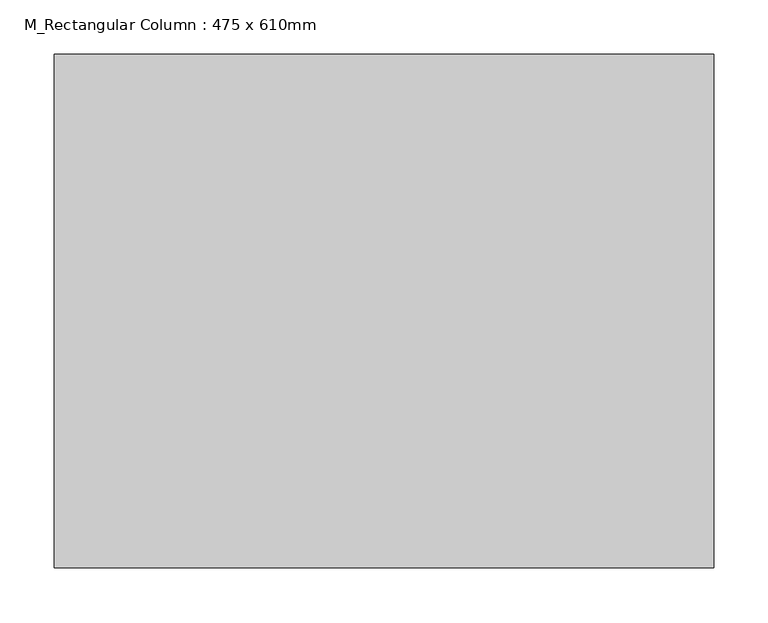
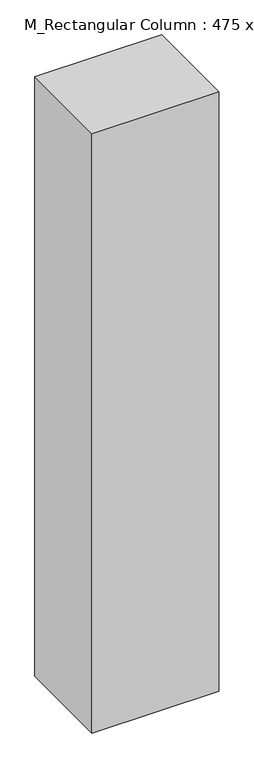
"""IFC4 building model written with IfcOpenShell, lengths in millimetres: column geometry, M_Rectangular Column : 475 x 610mm."""

from ifc_helpers import new_model, si_unit, origin, origin_with_axes, place, context, project, spatial, polyline, outline, extrude, source, transform, mapped, element, save


def m_rectangular_column_475_x_610mm_5ff218ee(model_context):
    return source(origin(), model_context, "Body", "SweptSolid", [
        extrude(outline(polyline([(305.0, 237.5), (305.0, -237.5), (-305.0, -237.5), (-305.0, 237.5), (305.0, 237.5)])), origin_with_axes(), (0.0, 0.0, 1.0), 3048.0),
    ])


if __name__ == "__main__":
    model = new_model("IFC4")
    model_context = context("Model", 3, world=origin())
    ifc_project = project(units=[si_unit("LENGTHUNIT", "METRE", prefix="MILLI")], contexts=[model_context])
    site = spatial("IfcSite", under=ifc_project)
    building = spatial("IfcBuilding", under=site)
    placement = place(None, origin())
    m_rectangular_column_475_x_610mm_shape = m_rectangular_column_475_x_610mm_5ff218ee(model_context)
    element("IfcColumn", 1, ObjectType="M_Rectangular Column : 475 x 610mm", at=placement, inside=building, context=model_context, shape_type="MappedRepresentation", body=[
        mapped(m_rectangular_column_475_x_610mm_shape, transform((0.0, 0.0, 0.0), x_axis=(1.0, 0.0, 0.0), y_axis=(0.0, 1.0, 0.0), z_axis=(0.0, 0.0, 1.0))),
    ])
    save(model, "model.ifc")

# Revit data of these elements
# Type "M_Rectangular Column : 475 x 610mm"
#   Depth = 475 mm
#   Offset Base = 0 mm
#   Offset Top = 0 mm
#   Width = 610 mm
#   Material = none
